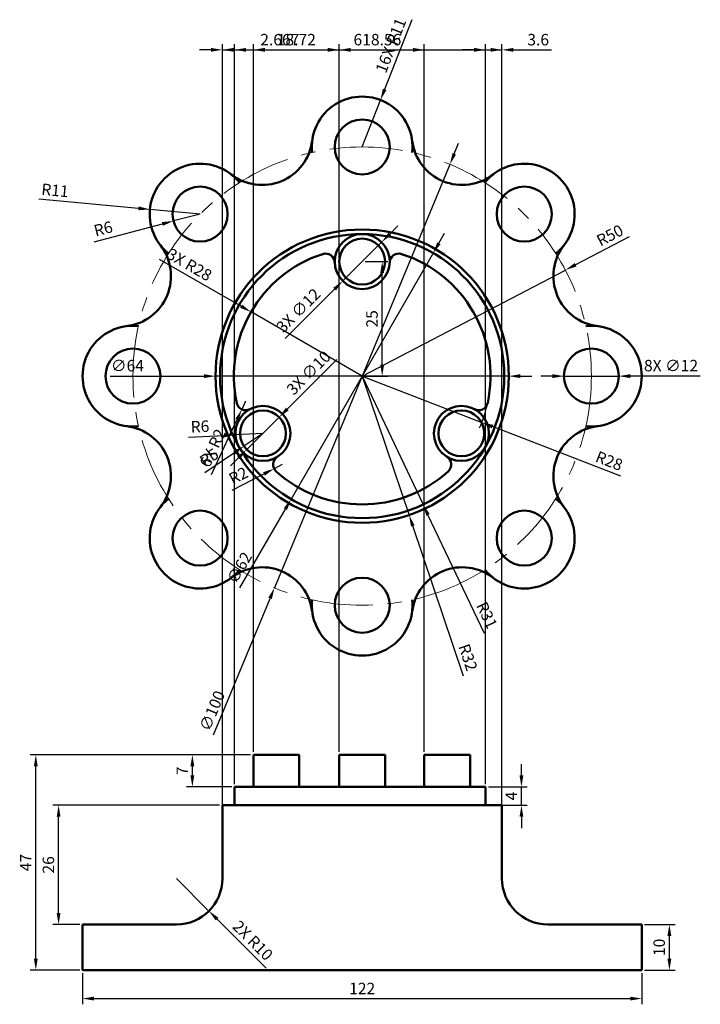
# Model space of a CAD drawing. Units: millimetres. Extents: x 2997 to 3145, y 1426 to 1641.
import ezdxf

# ---------------------------------------------------------------- set-up
doc = ezdxf.new("R2010")
doc.units = ezdxf.units.MM
doc.linetypes.add('CENTER', pattern=[50.8, 31.75, -6.35, 6.35, -6.35])
for name, color, linetype, lineweight in [('M-CNTR', 4, 'CENTER', 18), ('M-DIMS', 2, 'Continuous', 25), ('M-OUTL', 7, 'Continuous', 50)]:
    doc.layers.add(name, color=color, linetype=linetype, lineweight=lineweight)
doc.styles.get("Standard").update_dxf_attribs({"font": 'arial.ttf'})
doc.dimstyles.new('ISO-25', dxfattribs={"dimtxt": 2.5, "dimasz": 2.5, "dimexe": 1.25, "dimexo": 0.625, "dimtad": 1, "dimtxsty": 'Standard', "dimcen": 2.5, "dimadec": 0, "dimazin": 0, "dimtfac": 1, "dimtmove": 0, "dimatfit": 3, "dimfxl": 1, "dimarcsym": 0})

# ---------------------------------------------------------------- blocks, each defined once
blk = doc.blocks.new('*D1')
at = {"layer": 'Defpoints', "color": 0, "transparency": 16777216}
for p in [(3071.55, 1587.74), (3075.92, 1587.74), (3071.55, 1562.74)]:
    blk.add_point(p, dxfattribs=at)
at = {"layer": 'M-DIMS', "color": 0, "lineweight": -2, "transparency": 16777216}
for p, q in [((3072.18, 1587.74), (3077.17, 1587.74)), ((3075.92, 1565.24), (3075.92, 1585.24)), ((3072.18, 1562.74), (3077.17, 1562.74))]:
    blk.add_line(p, q, dxfattribs=at)
at = {"layer": 'M-DIMS', "color": 0, "transparency": 16777216}
for points in [[(3075.5, 1585.24), (3076.34, 1585.24), (3075.92, 1587.74)], [(3075.5, 1565.24), (3076.34, 1565.24), (3075.92, 1562.74)]]:
    blk.add_solid(points, dxfattribs=at)
at = {"layer": 'M-DIMS', "color": 0, "transparency": 16777216, "insert": (3074.02, 1575.24), "char_height": 2.5, "attachment_point": 5, "rotation": 90}
blk.add_mtext('25', dxfattribs=at)
blk = doc.blocks.new('*D2')
at = {"layer": 'Defpoints', "color": 0, "transparency": 16777216}
for p in [(3098.45, 1473.09), (3106.3, 1473.09), (3098.45, 1469.09)]:
    blk.add_point(p, dxfattribs=at)
at = {"layer": 'M-DIMS', "color": 0, "lineweight": -2, "transparency": 16777216}
for p, q in [((3106.3, 1475.59), (3106.3, 1478.09)), ((3099.08, 1473.09), (3107.55, 1473.09)), ((3106.3, 1469.09), (3106.3, 1473.09)), ((3099.08, 1469.09), (3107.55, 1469.09)), ((3106.3, 1466.59), (3106.3, 1464.09))]:
    blk.add_line(p, q, dxfattribs=at)
at = {"layer": 'M-DIMS', "color": 0, "transparency": 16777216}
for points in [[(3105.88, 1475.59), (3106.72, 1475.59), (3106.3, 1473.09)], [(3105.88, 1466.59), (3106.72, 1466.59), (3106.3, 1469.09)]]:
    blk.add_solid(points, dxfattribs=at)
at = {"layer": 'M-DIMS', "color": 0, "transparency": 16777216, "insert": (3104.42, 1471.09), "char_height": 2.5, "attachment_point": 5, "rotation": 90}
blk.add_mtext('4', dxfattribs=at)
blk = doc.blocks.new('*D3')
at = {"layer": 'Defpoints', "color": 0, "transparency": 16777216}
for p in [(3034.51, 1480.09), (3047.83, 1480.09), (3043.72, 1473.09)]:
    blk.add_point(p, dxfattribs=at)
at = {"layer": 'M-DIMS', "color": 0, "lineweight": -2, "transparency": 16777216}
for p, q in [((3047.21, 1480.09), (3033.26, 1480.09)), ((3034.51, 1475.59), (3034.51, 1477.59)), ((3043.09, 1473.09), (3033.26, 1473.09))]:
    blk.add_line(p, q, dxfattribs=at)
at = {"layer": 'M-DIMS', "color": 0, "transparency": 16777216}
for points in [[(3034.09, 1477.59), (3034.92, 1477.59), (3034.51, 1480.09)], [(3034.09, 1475.59), (3034.92, 1475.59), (3034.51, 1473.09)]]:
    blk.add_solid(points, dxfattribs=at)
at = {"layer": 'M-DIMS', "color": 0, "transparency": 16777216, "insert": (3032.63, 1476.59), "char_height": 2.5, "attachment_point": 5, "rotation": 90}
blk.add_mtext('7', dxfattribs=at)
blk = doc.blocks.new('*D4')
at = {"layer": 'Defpoints', "color": 0, "transparency": 16777216}
for p in [(3005.32, 1469.09), (3041.05, 1469.09), (3010.55, 1443.09)]:
    blk.add_point(p, dxfattribs=at)
at = {"layer": 'M-DIMS', "color": 0, "lineweight": -2, "transparency": 16777216}
for p, q in [((3040.43, 1469.09), (3004.07, 1469.09)), ((3005.32, 1445.59), (3005.32, 1466.59)), ((3009.93, 1443.09), (3004.07, 1443.09))]:
    blk.add_line(p, q, dxfattribs=at)
at = {"layer": 'M-DIMS', "color": 0, "transparency": 16777216}
for points in [[(3004.91, 1466.59), (3005.74, 1466.59), (3005.32, 1469.09)], [(3004.91, 1445.59), (3005.74, 1445.59), (3005.32, 1443.09)]]:
    blk.add_solid(points, dxfattribs=at)
at = {"layer": 'M-DIMS', "color": 0, "transparency": 16777216, "insert": (3003.42, 1456.09), "char_height": 2.5, "attachment_point": 5, "rotation": 90}
blk.add_mtext('26', dxfattribs=at)
blk = doc.blocks.new('*D5')
at = {"layer": 'Defpoints', "color": 0, "transparency": 16777216}
for p in [(3132.55, 1443.09), (3138.58, 1443.09), (3132.55, 1433.09)]:
    blk.add_point(p, dxfattribs=at)
at = {"layer": 'M-DIMS', "color": 0, "lineweight": -2, "transparency": 16777216}
for p, q in [((3133.18, 1443.09), (3139.83, 1443.09)), ((3138.58, 1435.59), (3138.58, 1440.59)), ((3133.18, 1433.09), (3139.83, 1433.09))]:
    blk.add_line(p, q, dxfattribs=at)
at = {"layer": 'M-DIMS', "color": 0, "transparency": 16777216}
for points in [[(3138.16, 1440.59), (3139, 1440.59), (3138.58, 1443.09)], [(3138.16, 1435.59), (3139, 1435.59), (3138.58, 1433.09)]]:
    blk.add_solid(points, dxfattribs=at)
at = {"layer": 'M-DIMS', "color": 0, "transparency": 16777216, "insert": (3136.68, 1438.09), "char_height": 2.5, "attachment_point": 5, "rotation": 90}
blk.add_mtext('10', dxfattribs=at)
blk = doc.blocks.new('*D6')
at = {"layer": 'Defpoints', "color": 0, "transparency": 16777216}
for p in [(3010.55, 1433.09), (3132.55, 1433.09), (3132.55, 1426.91)]:
    blk.add_point(p, dxfattribs=at)
at = {"layer": 'M-DIMS', "color": 0, "lineweight": -2, "transparency": 16777216}
for p, q in [((3010.55, 1432.47), (3010.55, 1425.66)), ((3132.55, 1432.47), (3132.55, 1425.66)), ((3013.05, 1426.91), (3130.05, 1426.91))]:
    blk.add_line(p, q, dxfattribs=at)
at = {"layer": 'M-DIMS', "color": 0, "transparency": 16777216}
for points in [[(3013.05, 1427.33), (3013.05, 1426.49), (3010.55, 1426.91)], [(3130.05, 1427.33), (3130.05, 1426.49), (3132.55, 1426.91)]]:
    blk.add_solid(points, dxfattribs=at)
at = {"layer": 'M-DIMS', "color": 0, "transparency": 16777216, "insert": (3071.55, 1428.79), "char_height": 2.5, "attachment_point": 5}
blk.add_mtext('122', dxfattribs=at)
blk = doc.blocks.new('*D7')
at = {"layer": 'Defpoints', "color": 0, "transparency": 16777216}
for p in [(3071.55, 1562.74), (3081.79, 1532.42)]:
    blk.add_point(p, dxfattribs=at)
at = {"layer": 'M-DIMS', "color": 0, "lineweight": -2, "transparency": 16777216}
for p, q in [((3071.55, 1562.74), (3081.79, 1532.42)), ((3093.68, 1497.24), (3082.59, 1530.05))]:
    blk.add_line(p, q, dxfattribs=at)
at = {"layer": 'M-DIMS', "color": 0, "transparency": 16777216}
blk.add_solid([(3082.99, 1530.19), (3082.2, 1529.92), (3081.79, 1532.42)], dxfattribs=at)
at = {"layer": 'M-DIMS', "color": 0, "transparency": 16777216, "insert": (3094.33, 1501.26), "char_height": 2.5, "attachment_point": 5, "rotation": 288.6639}
blk.add_mtext('R32', dxfattribs=at)
blk = doc.blocks.new('*D8')
at = {"layer": 'Defpoints', "color": 0, "transparency": 16777216}
for p in [(3071.55, 1562.74), (3084.84, 1534.73)]:
    blk.add_point(p, dxfattribs=at)
at = {"layer": 'M-DIMS', "color": 0, "lineweight": -2, "transparency": 16777216}
for p, q in [((3071.55, 1562.74), (3084.84, 1534.73)), ((3098.21, 1506.56), (3085.91, 1532.47))]:
    blk.add_line(p, q, dxfattribs=at)
at = {"layer": 'M-DIMS', "color": 0, "transparency": 16777216}
blk.add_solid([(3086.29, 1532.65), (3085.54, 1532.3), (3084.84, 1534.73)], dxfattribs=at)
at = {"layer": 'M-DIMS', "color": 0, "transparency": 16777216, "insert": (3098.48, 1510.42), "char_height": 2.5, "attachment_point": 5, "rotation": 295.3844}
blk.add_mtext('R31', dxfattribs=at)
blk = doc.blocks.new('*D9')
at = {"layer": 'Defpoints', "color": 0, "transparency": 16777216}
for p in [(3071.55, 1562.74), (3097.66, 1552.63)]:
    blk.add_point(p, dxfattribs=at)
at = {"layer": 'M-DIMS', "color": 0, "lineweight": -2, "transparency": 16777216}
for p, q in [((3071.55, 1562.74), (3097.66, 1552.63)), ((3128.01, 1540.88), (3099.99, 1551.73))]:
    blk.add_line(p, q, dxfattribs=at)
blk.add_arc((3071.55, 1562.74), 28, 336.2727, 346.6315, dxfattribs=at)
at = {"layer": 'M-DIMS', "color": 0, "transparency": 16777216}
blk.add_solid([(3100.15, 1552.11), (3099.84, 1551.34), (3097.66, 1552.63)], dxfattribs=at)
at = {"layer": 'M-DIMS', "color": 0, "transparency": 16777216, "insert": (3125.33, 1543.95), "char_height": 2.5, "attachment_point": 5, "rotation": 338.8306}
blk.add_mtext('R28', dxfattribs=at)
blk = doc.blocks.new('*D10')
at = {"layer": 'Defpoints', "color": 0, "transparency": 16777216}
for p in [(3043.91, 1549.93), (3049.9, 1550.24)]:
    blk.add_point(p, dxfattribs=at)
at = {"layer": 'M-DIMS', "color": 0, "lineweight": -2, "transparency": 16777216}
for p, q in [((3033.64, 1549.39), (3041.41, 1549.8)), ((3049.9, 1550.24), (3043.91, 1549.93))]:
    blk.add_line(p, q, dxfattribs=at)
at = {"layer": 'M-DIMS', "color": 0, "transparency": 16777216}
blk.add_solid([(3041.39, 1550.21), (3041.44, 1549.38), (3043.91, 1549.93)], dxfattribs=at)
at = {"layer": 'M-DIMS', "color": 0, "transparency": 16777216, "insert": (3036.18, 1551.43), "char_height": 2.5, "attachment_point": 5, "rotation": 2.9931}
blk.add_mtext('R6', dxfattribs=at)
blk = doc.blocks.new('*D11')
at = {"layer": 'Defpoints', "color": 0, "transparency": 16777216}
for p in [(3049.9, 1550.24), (3045.76, 1547.45)]:
    blk.add_point(p, dxfattribs=at)
at = {"layer": 'M-DIMS', "color": 0, "lineweight": -2, "transparency": 16777216}
for p, q in [((3049.9, 1550.24), (3045.76, 1547.45)), ((3037.21, 1541.69), (3043.68, 1546.05))]:
    blk.add_line(p, q, dxfattribs=at)
at = {"layer": 'M-DIMS', "color": 0, "transparency": 16777216}
blk.add_solid([(3043.45, 1546.4), (3043.91, 1545.7), (3045.76, 1547.45)], dxfattribs=at)
at = {"layer": 'M-DIMS', "color": 0, "transparency": 16777216, "insert": (3038.35, 1544.75), "char_height": 2.5, "attachment_point": 5, "rotation": 33.9573}
blk.add_mtext('R5', dxfattribs=at)
blk = doc.blocks.new('*D12')
at = {"layer": 'Defpoints', "color": 0, "transparency": 16777216}
for p in [(3054.13, 1543.45), (3052.34, 1542.54)]:
    blk.add_point(p, dxfattribs=at)
at = {"layer": 'M-DIMS', "color": 0, "lineweight": -2, "transparency": 16777216}
for p, q in [((3054.13, 1543.45), (3052.34, 1542.54)), ((3043.21, 1537.88), (3050.12, 1541.4))]:
    blk.add_line(p, q, dxfattribs=at)
at = {"layer": 'M-DIMS', "color": 0, "transparency": 16777216}
blk.add_solid([(3049.93, 1541.77), (3050.31, 1541.03), (3052.34, 1542.54)], dxfattribs=at)
at = {"layer": 'M-DIMS', "color": 0, "transparency": 16777216, "insert": (3044.69, 1540.75), "char_height": 2.5, "attachment_point": 5, "rotation": 27.0151}
blk.add_mtext('R2', dxfattribs=at)
blk = doc.blocks.new('*D13')
at = {"layer": 'Defpoints', "color": 0, "transparency": 16777216}
for p in [(3115.88, 1585.88), (3071.55, 1562.74)]:
    blk.add_point(p, dxfattribs=at)
at = {"layer": 'M-DIMS', "color": 0, "lineweight": -2, "transparency": 16777216}
for p, q in [((3129.83, 1593.17), (3118.09, 1587.04)), ((3071.55, 1562.74), (3115.88, 1585.88))]:
    blk.add_line(p, q, dxfattribs=at)
at = {"layer": 'M-DIMS', "color": 0, "transparency": 16777216}
blk.add_solid([(3117.9, 1587.41), (3118.28, 1586.67), (3115.88, 1585.88)], dxfattribs=at)
at = {"layer": 'M-DIMS', "color": 0, "transparency": 16777216, "insert": (3125.75, 1593.18), "char_height": 2.5, "attachment_point": 5, "rotation": 27.5701}
blk.add_mtext('R50', dxfattribs=at)
blk = doc.blocks.new('*D14')
at = {"layer": 'Defpoints', "color": 0, "transparency": 16777216}
for p in [(3030.39, 1596.59), (3036.2, 1598.1)]:
    blk.add_point(p, dxfattribs=at)
at = {"layer": 'M-DIMS', "color": 0, "lineweight": -2, "transparency": 16777216}
for p, q in [((3036.2, 1598.1), (3030.39, 1596.59)), ((3013.06, 1592.08), (3027.97, 1595.96))]:
    blk.add_line(p, q, dxfattribs=at)
at = {"layer": 'M-DIMS', "color": 0, "transparency": 16777216}
blk.add_solid([(3027.87, 1596.36), (3028.08, 1595.55), (3030.39, 1596.59)], dxfattribs=at)
at = {"layer": 'M-DIMS', "color": 0, "transparency": 16777216, "insert": (3015.14, 1594.59), "char_height": 2.5, "attachment_point": 5, "rotation": 14.567}
blk.add_mtext('R6', dxfattribs=at)
blk = doc.blocks.new('*D15')
at = {"layer": 'Defpoints', "color": 0, "transparency": 16777216}
for p in [(3025.25, 1599.12), (3036.2, 1598.1)]:
    blk.add_point(p, dxfattribs=at)
at = {"layer": 'M-DIMS', "color": 0, "lineweight": -2, "transparency": 16777216}
for p, q in [((3000.99, 1601.4), (3022.76, 1599.36)), ((3036.2, 1598.1), (3025.25, 1599.12))]:
    blk.add_line(p, q, dxfattribs=at)
at = {"layer": 'M-DIMS', "color": 0, "transparency": 16777216}
blk.add_solid([(3022.8, 1599.77), (3022.72, 1598.94), (3025.25, 1599.12)], dxfattribs=at)
at = {"layer": 'M-DIMS', "color": 0, "transparency": 16777216, "insert": (3004.52, 1602.96), "char_height": 2.5, "attachment_point": 5, "rotation": 354.6363}
blk.add_mtext('R11', dxfattribs=at)
blk = doc.blocks.new('MOUNTING-LUG-D12')
blk.add_circle((0, 0), 6)
blk.add_arc((0, 0), 11, 353.6847, 186.3153)
blk = doc.blocks.new('INNER-BOSS-D10')
for radius in [6, 5]:
    blk.add_circle((0, 0), radius)
for centre, start, end in [((-8, -0.26), 1.8624, 107.9104), ((8, -0.26), 72.0896, 178.1376)]:
    blk.add_arc(centre, 2, start, end)
blk = doc.blocks.new('BOSS-ELEVATION-10X7')
for p, q in [((-5, 0), (-5, 7)), ((-5, 7), (5, 7)), ((5, 7), (5, 0))]:
    blk.add_line(p, q)
blk = doc.blocks.new('*D19')
at = {"layer": 'Defpoints', "color": 0, "transparency": 16777216}
for p in [(3000.35, 1480.09), (3047.83, 1480.09), (3010.55, 1433.09)]:
    blk.add_point(p, dxfattribs=at)
at = {"layer": 'M-DIMS', "color": 0, "lineweight": -2, "transparency": 16777216}
for p, q in [((3047.21, 1480.09), (2999.1, 1480.09)), ((3000.35, 1435.59), (3000.35, 1477.59)), ((3009.93, 1433.09), (2999.1, 1433.09))]:
    blk.add_line(p, q, dxfattribs=at)
at = {"layer": 'M-DIMS', "color": 0, "transparency": 16777216}
for points in [[(2999.94, 1477.59), (3000.77, 1477.59), (3000.35, 1480.09)], [(2999.94, 1435.59), (3000.77, 1435.59), (3000.35, 1433.09)]]:
    blk.add_solid(points, dxfattribs=at)
at = {"layer": 'M-DIMS', "color": 0, "transparency": 16777216, "insert": (2998.48, 1456.59), "char_height": 2.5, "attachment_point": 5, "rotation": 90}
blk.add_mtext('47', dxfattribs=at)
blk = doc.blocks.new('*D20')
at = {"layer": 'Defpoints', "color": 0, "transparency": 16777216}
for p in [(3102.05, 1633.94), (3041.05, 1453.09), (3102.05, 1453.09)]:
    blk.add_point(p, dxfattribs=at)
at = {"layer": 'M-DIMS', "color": 0, "lineweight": -2, "transparency": 16777216}
for p, q in [((3041.05, 1453.72), (3041.05, 1635.19)), ((3102.05, 1453.72), (3102.05, 1635.19)), ((3043.55, 1633.94), (3099.55, 1633.94))]:
    blk.add_line(p, q, dxfattribs=at)
at = {"layer": 'M-DIMS', "color": 0, "transparency": 16777216}
for points in [[(3043.55, 1634.36), (3043.55, 1633.52), (3041.05, 1633.94)], [(3099.55, 1634.36), (3099.55, 1633.52), (3102.05, 1633.94)]]:
    blk.add_solid(points, dxfattribs=at)
at = {"layer": 'M-DIMS', "color": 0, "transparency": 16777216, "insert": (3071.55, 1635.84), "char_height": 2.5, "attachment_point": 5}
blk.add_mtext('61', dxfattribs=at)
blk = doc.blocks.new('*D21')
at = {"layer": 'Defpoints', "color": 0, "transparency": 16777216}
for p in [(3066.55, 1633.94), (3047.83, 1480.09), (3066.55, 1480.09)]:
    blk.add_point(p, dxfattribs=at)
at = {"layer": 'M-DIMS', "color": 0, "lineweight": -2, "transparency": 16777216}
for p, q in [((3047.83, 1480.72), (3047.83, 1635.19)), ((3066.55, 1480.72), (3066.55, 1635.19)), ((3050.33, 1633.94), (3064.05, 1633.94))]:
    blk.add_line(p, q, dxfattribs=at)
at = {"layer": 'M-DIMS', "color": 0, "transparency": 16777216}
for points in [[(3050.33, 1634.36), (3050.33, 1633.52), (3047.83, 1633.94)], [(3064.05, 1634.36), (3064.05, 1633.52), (3066.55, 1633.94)]]:
    blk.add_solid(points, dxfattribs=at)
at = {"layer": 'M-DIMS', "color": 0, "transparency": 16777216, "insert": (3057.19, 1635.84), "char_height": 2.5, "attachment_point": 5}
blk.add_mtext('18.72', dxfattribs=at)
blk = doc.blocks.new('*D22')
at = {"layer": 'Defpoints', "color": 0, "transparency": 16777216}
for p in [(3085.11, 1633.94), (3066.55, 1480.09), (3085.11, 1480.09)]:
    blk.add_point(p, dxfattribs=at)
at = {"layer": 'M-DIMS', "color": 0, "lineweight": -2, "transparency": 16777216}
for p, q in [((3066.55, 1480.72), (3066.55, 1635.19)), ((3085.11, 1480.72), (3085.11, 1635.19)), ((3069.05, 1633.94), (3082.61, 1633.94))]:
    blk.add_line(p, q, dxfattribs=at)
at = {"layer": 'M-DIMS', "color": 0, "transparency": 16777216}
for points in [[(3069.05, 1634.36), (3069.05, 1633.52), (3066.55, 1633.94)], [(3082.61, 1634.36), (3082.61, 1633.52), (3085.11, 1633.94)]]:
    blk.add_solid(points, dxfattribs=at)
at = {"layer": 'M-DIMS', "color": 0, "transparency": 16777216, "insert": (3075.83, 1635.84), "char_height": 2.5, "attachment_point": 5}
blk.add_mtext('18.56', dxfattribs=at)
blk = doc.blocks.new('*D23')
at = {"layer": 'Defpoints', "color": 0, "transparency": 16777216}
for p in [(3043.72, 1633.94), (3043.72, 1473.09), (3041.05, 1469.09)]:
    blk.add_point(p, dxfattribs=at)
at = {"layer": 'M-DIMS', "color": 0, "lineweight": -2, "transparency": 16777216}
for p, q in [((3041.05, 1469.72), (3041.05, 1635.19)), ((3043.72, 1473.72), (3043.72, 1635.19)), ((3038.55, 1633.94), (3036.05, 1633.94)), ((3041.05, 1633.94), (3043.72, 1633.94)), ((3046.22, 1633.94), (3058.45, 1633.94))]:
    blk.add_line(p, q, dxfattribs=at)
at = {"layer": 'M-DIMS', "color": 0, "transparency": 16777216}
for points in [[(3038.55, 1634.36), (3038.55, 1633.52), (3041.05, 1633.94)], [(3046.22, 1634.36), (3046.22, 1633.52), (3043.72, 1633.94)]]:
    blk.add_solid(points, dxfattribs=at)
at = {"layer": 'M-DIMS', "color": 0, "transparency": 16777216, "insert": (3053.58, 1635.84), "char_height": 2.5, "attachment_point": 5}
blk.add_mtext('2.667', dxfattribs=at)
blk = doc.blocks.new('*D24')
at = {"layer": 'Defpoints', "color": 0, "transparency": 16777216}
for p in [(3102.05, 1633.94), (3098.45, 1473.09), (3102.05, 1469.09)]:
    blk.add_point(p, dxfattribs=at)
at = {"layer": 'M-DIMS', "color": 0, "lineweight": -2, "transparency": 16777216}
for p, q in [((3098.45, 1473.72), (3098.45, 1635.19)), ((3102.05, 1469.72), (3102.05, 1635.19)), ((3095.95, 1633.94), (3093.45, 1633.94)), ((3098.45, 1633.94), (3102.05, 1633.94)), ((3104.55, 1633.94), (3112.85, 1633.94))]:
    blk.add_line(p, q, dxfattribs=at)
at = {"layer": 'M-DIMS', "color": 0, "transparency": 16777216}
for points in [[(3095.95, 1634.36), (3095.95, 1633.52), (3098.45, 1633.94)], [(3104.55, 1634.36), (3104.55, 1633.52), (3102.05, 1633.94)]]:
    blk.add_solid(points, dxfattribs=at)
at = {"layer": 'M-DIMS', "color": 0, "transparency": 16777216, "insert": (3109.95, 1635.84), "char_height": 2.5, "attachment_point": 5}
blk.add_mtext('3.6', dxfattribs=at)
blk = doc.blocks.new('*D25')
at = {"layer": 'Defpoints', "color": 0, "transparency": 16777216}
for p in [(3031.05, 1453.09), (3038.12, 1446.02)]:
    blk.add_point(p, dxfattribs=at)
at = {"layer": 'M-DIMS', "color": 0, "lineweight": -2, "transparency": 16777216}
for p, q in [((3031.05, 1453.09), (3038.12, 1446.02)), ((3050.59, 1433.55), (3039.89, 1444.25))]:
    blk.add_line(p, q, dxfattribs=at)
at = {"layer": 'M-DIMS', "color": 0, "transparency": 16777216}
blk.add_solid([(3040.19, 1444.55), (3039.6, 1443.96), (3038.12, 1446.02)], dxfattribs=at)
at = {"layer": 'M-DIMS', "color": 0, "transparency": 16777216, "insert": (3047.47, 1439.36), "char_height": 2.5, "attachment_point": 5, "rotation": 314.9999}
blk.add_mtext('2X R10', dxfattribs=at)
blk = doc.blocks.new('*D26')
at = {"layer": 'Defpoints', "color": 0, "transparency": 16777216}
for p in [(3090.69, 1608.93), (3052.42, 1516.55)]:
    blk.add_point(p, dxfattribs=at)
at = {"layer": 'M-DIMS', "color": 0, "lineweight": -2, "transparency": 16777216}
for p, q in [((3091.64, 1611.24), (3092.6, 1613.55)), ((3090.69, 1608.93), (3052.42, 1516.55)), ((3039.12, 1484.45), (3051.46, 1514.24))]:
    blk.add_line(p, q, dxfattribs=at)
at = {"layer": 'M-DIMS', "color": 0, "transparency": 16777216}
for points in [[(3091.26, 1611.4), (3092.03, 1611.08), (3090.69, 1608.93)], [(3051.08, 1514.4), (3051.85, 1514.08), (3052.42, 1516.55)]]:
    blk.add_solid(points, dxfattribs=at)
at = {"layer": 'M-DIMS', "color": 0, "transparency": 16777216, "insert": (3039.12, 1489.58), "char_height": 2.5, "attachment_point": 5, "rotation": 67.5002}
blk.add_mtext('∅100', dxfattribs=at)
blk = doc.blocks.new('*D27')
at = {"layer": 'Defpoints', "color": 0, "transparency": 16777216}
for p in [(3115.55, 1562.74), (3127.55, 1562.74)]:
    blk.add_point(p, dxfattribs=at)
at = {"layer": 'M-DIMS', "color": 0, "lineweight": -2, "transparency": 16777216}
for p, q in [((3113.05, 1562.74), (3110.55, 1562.74)), ((3115.55, 1562.74), (3127.55, 1562.74)), ((3145.32, 1562.74), (3130.05, 1562.74))]:
    blk.add_line(p, q, dxfattribs=at)
at = {"layer": 'M-DIMS', "color": 0, "transparency": 16777216}
for points in [[(3113.05, 1563.16), (3113.05, 1562.32), (3115.55, 1562.74)], [(3130.05, 1563.16), (3130.05, 1562.32), (3127.55, 1562.74)]]:
    blk.add_solid(points, dxfattribs=at)
at = {"layer": 'M-DIMS', "color": 0, "transparency": 16777216, "insert": (3138.94, 1564.71), "char_height": 2.5, "attachment_point": 5, "rotation": 0.0009}
blk.add_mtext('8X ∅12', dxfattribs=at)
blk = doc.blocks.new('*D28')
at = {"layer": 'Defpoints', "color": 0, "transparency": 16777216}
for p in [(3075.55, 1622.99), (3071.55, 1612.74)]:
    blk.add_point(p, dxfattribs=at)
at = {"layer": 'M-DIMS', "color": 0, "lineweight": -2, "transparency": 16777216}
for p, q in [((3082.4, 1640.52), (3076.46, 1625.32)), ((3071.55, 1612.74), (3075.55, 1622.99))]:
    blk.add_line(p, q, dxfattribs=at)
at = {"layer": 'M-DIMS', "color": 0, "transparency": 16777216}
blk.add_solid([(3076.07, 1625.47), (3076.85, 1625.16), (3075.55, 1622.99)], dxfattribs=at)
at = {"layer": 'M-DIMS', "color": 0, "transparency": 16777216, "insert": (3078.11, 1634.77), "char_height": 2.5, "attachment_point": 5, "rotation": 68.6764}
blk.add_mtext('16X R11', dxfattribs=at)
blk = doc.blocks.new('*D29')
at = {"layer": 'Defpoints', "color": 0, "transparency": 16777216}
for p in [(3039.55, 1562.74), (3103.55, 1562.74)]:
    blk.add_point(p, dxfattribs=at)
at = {"layer": 'M-DIMS', "color": 0, "lineweight": -2, "transparency": 16777216}
for p, q in [((3016.58, 1562.74), (3037.05, 1562.74)), ((3103.55, 1562.74), (3039.55, 1562.74)), ((3106.05, 1562.74), (3108.55, 1562.74))]:
    blk.add_line(p, q, dxfattribs=at)
at = {"layer": 'M-DIMS', "color": 0, "transparency": 16777216}
for points in [[(3037.05, 1563.16), (3037.05, 1562.32), (3039.55, 1562.74)], [(3106.05, 1563.16), (3106.05, 1562.32), (3103.55, 1562.74)]]:
    blk.add_solid(points, dxfattribs=at)
at = {"layer": 'M-DIMS', "color": 0, "transparency": 16777216, "insert": (3020.35, 1564.71), "char_height": 2.5, "attachment_point": 5, "rotation": 359.9998}
blk.add_mtext('∅64', dxfattribs=at)
blk = doc.blocks.new('*D30')
at = {"layer": 'Defpoints', "color": 0, "transparency": 16777216}
for p in [(3087.05, 1589.59), (3056.05, 1535.89)]:
    blk.add_point(p, dxfattribs=at)
at = {"layer": 'M-DIMS', "color": 0, "lineweight": -2, "transparency": 16777216}
for p, q in [((3088.3, 1591.75), (3089.55, 1593.92)), ((3087.05, 1589.59), (3056.05, 1535.89)), ((3044.87, 1516.53), (3054.8, 1533.73))]:
    blk.add_line(p, q, dxfattribs=at)
at = {"layer": 'M-DIMS', "color": 0, "transparency": 16777216}
for points in [[(3087.94, 1591.96), (3088.66, 1591.54), (3087.05, 1589.59)], [(3054.44, 1533.94), (3055.16, 1533.52), (3056.05, 1535.89)]]:
    blk.add_solid(points, dxfattribs=at)
at = {"layer": 'M-DIMS', "color": 0, "transparency": 16777216, "insert": (3045.05, 1520.77), "char_height": 2.5, "attachment_point": 5, "rotation": 60.0002}
blk.add_mtext('∅62', dxfattribs=at)
blk = doc.blocks.new('*D31')
at = {"layer": 'Defpoints', "color": 0, "transparency": 16777216}
for p in [(3047.3, 1576.74), (3071.55, 1562.74)]:
    blk.add_point(p, dxfattribs=at)
at = {"layer": 'M-DIMS', "color": 0, "lineweight": -2, "transparency": 16777216}
for p, q in [((3027.3, 1588.29), (3045.14, 1577.99)), ((3071.55, 1562.74), (3047.3, 1576.74))]:
    blk.add_line(p, q, dxfattribs=at)
at = {"layer": 'M-DIMS', "color": 0, "transparency": 16777216}
blk.add_solid([(3045.35, 1578.35), (3044.93, 1577.63), (3047.3, 1576.74)], dxfattribs=at)
at = {"layer": 'M-DIMS', "color": 0, "transparency": 16777216, "insert": (3033.71, 1586.79), "char_height": 2.5, "attachment_point": 5, "rotation": 330.0001}
blk.add_mtext('3X R28', dxfattribs=at)
blk = doc.blocks.new('*D32')
at = {"layer": 'Defpoints', "color": 0, "transparency": 16777216}
for p in [(3046.13, 1557.29), (3045.29, 1555.48)]:
    blk.add_point(p, dxfattribs=at)
at = {"layer": 'M-DIMS', "color": 0, "lineweight": -2, "transparency": 16777216}
for p, q in [((3046.13, 1557.29), (3045.29, 1555.48)), ((3038.71, 1541.29), (3044.24, 1553.21))]:
    blk.add_line(p, q, dxfattribs=at)
at = {"layer": 'M-DIMS', "color": 0, "transparency": 16777216}
blk.add_solid([(3043.86, 1553.39), (3044.61, 1553.04), (3045.29, 1555.48)], dxfattribs=at)
at = {"layer": 'M-DIMS', "color": 0, "transparency": 16777216, "insert": (3039.22, 1546.92), "char_height": 2.5, "attachment_point": 5, "rotation": 65.1163}
blk.add_mtext('6X R2', dxfattribs=at)
blk = doc.blocks.new('*D33')
at = {"layer": 'Defpoints', "color": 0, "transparency": 16777216}
for p in [(3053.44, 1553.78), (3046.37, 1546.7)]:
    blk.add_point(p, dxfattribs=at)
at = {"layer": 'M-DIMS', "color": 0, "lineweight": -2, "transparency": 16777216}
for p, q in [((3066.01, 1566.35), (3055.21, 1555.54)), ((3046.37, 1546.7), (3053.44, 1553.78)), ((3044.6, 1544.94), (3042.83, 1543.17))]:
    blk.add_line(p, q, dxfattribs=at)
at = {"layer": 'M-DIMS', "color": 0, "transparency": 16777216}
for points in [[(3054.91, 1555.84), (3055.5, 1555.25), (3053.44, 1553.78)], [(3044.3, 1545.23), (3044.89, 1544.64), (3046.37, 1546.7)]]:
    blk.add_solid(points, dxfattribs=at)
at = {"layer": 'M-DIMS', "color": 0, "transparency": 16777216, "insert": (3060.1, 1563.22), "char_height": 2.5, "attachment_point": 5, "rotation": 45.0035}
blk.add_mtext('3X ∅10', dxfattribs=at)
blk = doc.blocks.new('*D34')
at = {"layer": 'Defpoints', "color": 0, "transparency": 16777216}
for p in [(3075.8, 1591.98), (3067.31, 1583.5)]:
    blk.add_point(p, dxfattribs=at)
at = {"layer": 'M-DIMS', "color": 0, "lineweight": -2, "transparency": 16777216}
for p, q in [((3077.56, 1593.75), (3079.33, 1595.52)), ((3075.8, 1591.98), (3067.31, 1583.5)), ((3054.75, 1570.94), (3065.54, 1581.73))]:
    blk.add_line(p, q, dxfattribs=at)
at = {"layer": 'M-DIMS', "color": 0, "transparency": 16777216}
for points in [[(3077.27, 1594.04), (3077.86, 1593.45), (3075.8, 1591.98)], [(3065.25, 1582.02), (3065.84, 1581.44), (3067.31, 1583.5)]]:
    blk.add_solid(points, dxfattribs=at)
at = {"layer": 'M-DIMS', "color": 0, "transparency": 16777216, "insert": (3057.87, 1576.85), "char_height": 2.5, "attachment_point": 5, "rotation": 44.9928}
blk.add_mtext('3X ∅12', dxfattribs=at)

msp = doc.modelspace()

# ---------------------------------------------------------------- linework, layer by layer
at = {"layer": 'M-CNTR', "ltscale": 0.5}
msp.add_circle((3071.553, 1562.7399), 50, dxfattribs=at)
at = {"layer": 'M-OUTL'}
for p, q in [((3043.7198, 1469.0921), (3043.7198, 1473.0921)), ((3098.4532, 1473.0921), (3043.7198, 1473.0921)), ((3098.4532, 1469.0921), (3098.4532, 1473.0921)), ((3041.053, 1453.0921), (3041.053, 1469.0921)), ((3041.053, 1469.0921), (3071.553, 1469.0921)), ((3102.053, 1469.0921), (3071.553, 1469.0921)), ((3102.053, 1453.0921), (3102.053, 1469.0921)), ((3010.553, 1433.0921), (3010.553, 1443.0921)), ((3031.053, 1443.0921), (3010.553, 1443.0921)), ((3132.553, 1443.0921), (3112.053, 1443.0921)), ((3132.553, 1433.0921), (3132.553, 1443.0921)), ((3071.553, 1433.0921), (3010.553, 1433.0921)), ((3071.553, 1433.0921), (3132.553, 1433.0921))]:
    msp.add_line(p, q, dxfattribs=at)
for radius in [32, 31]:
    msp.add_circle((3071.553, 1562.7399), radius, dxfattribs=at)
for centre, radius, start, end in [((3049.7203, 1615.4485), 11, 232.072132, 352.927868), ((3093.3856, 1615.4485), 11, 187.072132, 307.927868), ((3018.8444, 1584.5725), 11, 277.072132, 37.927868), ((3124.2616, 1584.5725), 11, 142.072132, 262.927868), ((3071.553, 1562.7399), 28, 107.910426, 192.089574), ((3071.553, 1562.7399), 28, 347.910426, 72.089574), ((3018.8444, 1540.9073), 11, 322.072132, 82.927868), ((3124.2616, 1540.9073), 11, 97.072132, 217.927868), ((3071.553, 1562.7399), 28, 227.910426, 312.089574), ((3049.7203, 1510.0313), 11, 7.072132, 127.927868), ((3093.3856, 1510.0313), 11, 52.072132, 172.927868), ((3031.053, 1453.0921), 10, 270, 0), ((3112.053, 1453.0921), 10, 180, 270)]:
    msp.add_arc(centre, radius, start, end, dxfattribs=at)

# ---------------------------------------------------------------- block references
for name, p in [('MOUNTING-LUG-D12', (3071.553, 1612.7399)), ('INNER-BOSS-D10', (3071.553, 1587.7399)), ('BOSS-ELEVATION-10X7', (3052.8313, 1473.0921)), ('BOSS-ELEVATION-10X7', (3071.553, 1473.0921)), ('BOSS-ELEVATION-10X7', (3090.1127, 1473.0921))]:
    msp.add_blockref(name, p, dxfattribs=at)
for name, p, rotation in [('MOUNTING-LUG-D12', (3036.1976, 1598.0952), 45.00000000000006), ('MOUNTING-LUG-D12', (3106.9083, 1598.0952), 314.9999999999966), ('MOUNTING-LUG-D12', (3021.553, 1562.7399), 89.99999999999991), ('MOUNTING-LUG-D12', (3121.553, 1562.7399), 269.9999999999977), ('INNER-BOSS-D10', (3049.9023, 1550.2399), 120.0000000000021), ('INNER-BOSS-D10', (3093.2036, 1550.2399), 239.9999999999982), ('MOUNTING-LUG-D12', (3036.1976, 1527.3846), 134.9999999999991), ('MOUNTING-LUG-D12', (3106.9083, 1527.3846), 224.9999999999994), ('MOUNTING-LUG-D12', (3071.553, 1512.7399), 180)]:
    msp.add_blockref(name, p, dxfattribs=dict(at, rotation=rotation))

# ---------------------------------------------------------------- dimensions: what is measured, and where the dimension line sits
at = {"layer": 'M-DIMS'}
for center, mpoint, text, picture, middle in [((3071.553, 1612.7399), (3075.5529, 1622.9869), '16X <>', '*D28', (3078.1126, 1634.7729)), ((3046.1296, 1557.2944), (3045.2881, 1555.4801), '6X <>', '*D32', (3039.2205, 1546.9177)), ((3031.053, 1453.0921), (3038.124, 1446.021), '2X <>', '*D25', (3047.4693, 1439.3647))]:
    dim = msp.add_radius_dim(center=center, mpoint=mpoint, text=text, dimstyle='ISO-25', override={"dimdec": 0, "dimlfac": 1, "dimrnd": 0, "dimzin": 0, "dimdsep": 46, "dimlunit": 2}, dxfattribs=at)
    dim.commit()
    dim.dimension.update_dxf_attribs({"geometry": picture, "text_midpoint": middle})
for base, p1, p2, override, picture, middle in [((3043.7198, 1633.9399), (3041.053, 1469.0921), (3043.7198, 1473.0921), {"dimdec": 3, "dimlfac": 1, "dimrnd": 0, "dimzin": 0, "dimdsep": 46, "dimlunit": 2}, '*D23', (3053.5843, 1635.8413)), ((3102.053, 1633.9399), (3041.053, 1453.0921), (3102.053, 1453.0921), {"dimdec": 0, "dimlfac": 1, "dimrnd": 0, "dimzin": 0, "dimdsep": 46, "dimlunit": 2}, '*D20', (3071.553, 1635.8413)), ((3066.553, 1633.9399), (3047.8313, 1480.0921), (3066.553, 1480.0921), {"dimdec": 2, "dimlfac": 1, "dimrnd": 0, "dimzin": 0, "dimdsep": 46, "dimlunit": 2}, '*D21', (3057.1921, 1635.8413)), ((3085.1127, 1633.9399), (3066.553, 1480.0921), (3085.1127, 1480.0921), {"dimdec": 2, "dimlfac": 1, "dimrnd": 0, "dimzin": 0, "dimdsep": 46, "dimlunit": 2}, '*D22', (3075.8328, 1635.8413)), ((3102.053, 1633.9399), (3098.4532, 1473.0921), (3102.053, 1469.0921), {"dimdec": 1, "dimlfac": 1, "dimrnd": 0, "dimzin": 0, "dimdsep": 46, "dimlunit": 2}, '*D24', (3109.952, 1635.8422)), ((3132.553, 1426.9099), (3010.553, 1433.0921), (3132.553, 1433.0921), {"dimclrd": 0, "dimclre": 0, "dimclrt": 0}, '*D6', (3071.553, 1428.79))]:
    dim = msp.add_linear_dim(base=base, p1=p1, p2=p2, dimstyle='ISO-25', override=override, dxfattribs=at)
    dim.commit()
    dim.dimension.update_dxf_attribs({"geometry": picture, "text_midpoint": middle})
for p1, p2, picture, middle in [((3090.687, 1608.9339), (3052.4189, 1516.5459), '*D26', (3040.9385, 1488.8294)), ((3087.0529, 1589.5867), (3056.053, 1535.8931), '*D30', (3046.7531, 1519.785)), ((3103.553, 1562.7398), (3039.553, 1562.74), '*D29', (3020.353, 1562.7401))]:
    dim = msp.add_diameter_dim_2p(p1=p1, p2=p2, dimstyle='ISO-25', override={"dimdec": 0, "dimlfac": 1, "dimrnd": 0, "dimzin": 0, "dimdsep": 46, "dimlunit": 2}, dxfattribs=at)
    dim.commit()
    dim.dimension.update_dxf_attribs({"geometry": picture, "text_midpoint": middle, "dimtype": 163})
for center, mpoint, picture, middle in [((3036.1976, 1598.0952), (3025.2458, 1599.1235), '*D15', (3004.3471, 1601.0856)), ((3036.1976, 1598.0952), (3030.3905, 1596.5862), '*D14', (3015.6153, 1592.7466)), ((3071.553, 1562.7399), (3115.8752, 1585.8815), '*D13', (3126.628, 1591.4958)), ((3071.553, 1562.7399), (3081.7935, 1532.4227), '*D7', (3092.5262, 1500.6485)), ((3071.553, 1562.7399), (3084.8423, 1534.7329), '*D8', (3096.7648, 1509.6064)), ((3071.553, 1562.7399), (3097.6634, 1552.6283), '*D9', (3124.6419, 1542.1806))]:
    dim = msp.add_radius_dim(center=center, mpoint=mpoint, dimstyle='ISO-25', override={"dimclrd": 0, "dimclre": 0, "dimclrt": 0}, dxfattribs=at)
    dim.commit()
    dim.dimension.update_dxf_attribs({"geometry": picture, "text_midpoint": middle, "dimtype": 164})
for p1, p2, text, picture, middle in [((3075.7961, 1591.982), (3067.3098, 1583.4978), '3X <>', '*D34', (3059.261, 1575.451)), ((3115.553, 1562.7398), (3127.553, 1562.74), '8X <>', '*D27', (3138.9368, 1562.7402))]:
    dim = msp.add_diameter_dim_2p(p1=p1, p2=p2, text=text, dimstyle='ISO-25', override={"dimdec": 0, "dimlfac": 1, "dimrnd": 0, "dimzin": 0, "dimdsep": 46, "dimlunit": 2}, dxfattribs=at)
    dim.commit()
    dim.dimension.update_dxf_attribs({"geometry": picture, "text_midpoint": middle})
dim = msp.add_radius_dim(center=(3071.553, 1562.7399), mpoint=(3047.3042, 1576.7399), text='3X <>', dimstyle='ISO-25', override={"dimdec": 0, "dimlfac": 1, "dimrnd": 0, "dimzin": 0, "dimdsep": 46, "dimlunit": 2}, dxfattribs=at)
dim.commit()
dim.dimension.update_dxf_attribs({"geometry": '*D31', "text_midpoint": (3032.755, 1585.1398), "dimtype": 164})
for base, p1, p2, override, picture, middle in [((3075.919, 1587.7399), (3071.553, 1562.7399), (3071.553, 1587.7399), {"dimclrd": 0, "dimclre": 0, "dimclrt": 0}, '*D1', (3074.0176, 1575.2399)), ((3000.353, 1480.0921), (3010.553, 1433.0921), (3047.8313, 1480.0921), {"dimdec": 0, "dimlfac": 1, "dimrnd": 0, "dimzin": 0, "dimdsep": 46, "dimlunit": 2}, '*D19', (2998.478, 1456.5921)), ((3034.5058, 1480.0921), (3043.7198, 1473.0921), (3047.8313, 1480.0921), {"dimclrd": 0, "dimclre": 0, "dimclrt": 0}, '*D3', (3032.6308, 1476.5921)), ((3106.299, 1473.0921), (3098.4532, 1469.0921), (3098.4532, 1473.0921), {"dimclrd": 0, "dimclre": 0, "dimclrt": 0}, '*D2', (3104.424, 1471.0921)), ((3005.3237, 1469.0921), (3010.553, 1443.0921), (3041.053, 1469.0921), {"dimclrd": 0, "dimclre": 0, "dimclrt": 0}, '*D4', (3003.4223, 1456.0921)), ((3138.5802, 1443.0921), (3132.553, 1433.0921), (3132.553, 1443.0921), {"dimclrd": 0, "dimclre": 0, "dimclrt": 0}, '*D5', (3136.6787, 1438.0921))]:
    dim = msp.add_linear_dim(base=base, p1=p1, p2=p2, angle=90, dimstyle='ISO-25', override=override, dxfattribs=at)
    dim.commit()
    dim.dimension.update_dxf_attribs({"geometry": picture, "text_midpoint": middle})
dim = msp.add_diameter_dim_2p(p1=(3046.367, 1546.7042), p2=(3053.4377, 1553.7757), text='3X <>', dimstyle='ISO-25', override={"dimdec": 0, "dimlfac": 1, "dimrnd": 0, "dimzin": 0, "dimdsep": 46, "dimlunit": 2}, dxfattribs=at)
dim.commit()
dim.dimension.update_dxf_attribs({"geometry": '*D33', "text_midpoint": (3061.491, 1561.83), "dimtype": 163})
for center, mpoint, picture, middle in [((3049.9023, 1550.2399), (3043.9105, 1549.9266), '*D10', (3036.1818, 1551.4265)), ((3049.9023, 1550.2399), (3045.7551, 1547.447), '*D11', (3038.3504, 1544.7468)), ((3054.1254, 1543.4454), (3052.3436, 1542.5369), '*D12', (3044.694, 1540.7471))]:
    dim = msp.add_radius_dim(center=center, mpoint=mpoint, dimstyle='ISO-25', override={"dimclrd": 0, "dimclre": 0, "dimclrt": 0}, dxfattribs=at)
    dim.commit()
    dim.dimension.update_dxf_attribs({"geometry": picture, "text_midpoint": middle})

doc.saveas('drawing.dxf')
